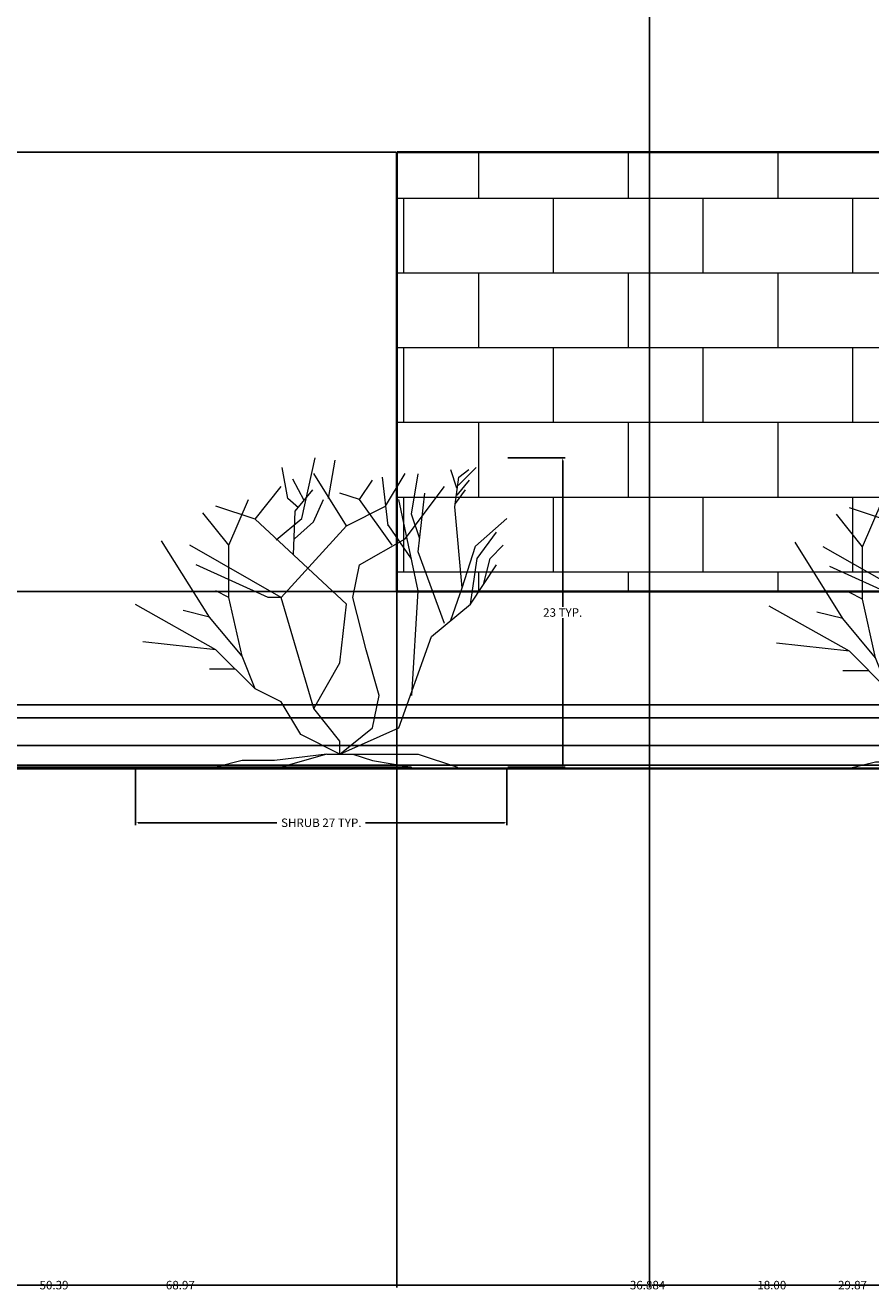
# Model space of a CAD drawing. Units: inches. Extents: x -13 to 809, y 112 to 656.
# Tile 2 of 55: x 49 to 111, y 112 to 205. Entities that reach past the tile are written whole.
import ezdxf

# ---------------------------------------------------------------- set-up
doc = ezdxf.new("R2010")
doc.units = ezdxf.units.IN
doc.header["$MEASUREMENT"] = 0
for name, color, linetype, lineweight in [('A-ANNO-DIMS', 2, 'Continuous', 18), ('A-ELEV', 7, 'Continuous', 35), ('A-ELEV-PATT', 8, 'Continuous', 13), ('L-PLNT', 3, 'Continuous', 18)]:
    doc.layers.add(name, color=color, linetype=linetype, lineweight=lineweight)
doc.styles.get("Standard").update_dxf_attribs({"font": 'arial.ttf'})
doc.dimstyles.get("Standard").update_dxf_attribs({"dimtxt": 0.625, "dimasz": 0.18, "dimexe": 0.18, "dimexo": 0.0625, "dimgap": 0.09, "dimtad": 0, "dimtih": 1, "dimtoh": 1, "dimdec": 4, "dimzin": 0, "dimdsep": 46, "dimlunit": 4, "dimtxsty": 'Standard', "dimcen": 0.09, "dimadec": 0, "dimazin": 0, "dimtfac": 1, "dimtdec": 4, "dimtofl": 0, "dimtmove": 0, "dimatfit": 3, "dimfxl": 1, "dimtolj": 1, "dimtzin": 0, "dimarcsym": 0})

# ---------------------------------------------------------------- blocks, each defined once
blk = doc.blocks.new('Shrub - elevation')
for p, q in [((-11.433, 18.289), (-10.457, 22.749)), ((-9.48, 19.775), (-8.992, 22.592)), ((-12.471, 19.775), (-12.898, 22.044)), ((-8.16, 17.76), (-10.56, 21.6)), ((-5.28, 19.2), (-3.84, 21.6)), ((-3.377, 18.602), (-2.888, 21.575)), ((-0.508, 21.888), (-0.081, 20.558)), ((0.041, 20.714), (1.384, 22.044)), ((0.102, 21.34), (0.835, 21.888)), ((-14.88, 18.24), (-12.96, 20.64)), ((-11.28, 19.619), (-12.104, 21.184)), ((-7.2, 19.68), (-6.24, 21.12)), ((-5.086, 17.741), (-5.513, 21.34)), ((-3.84, 16.8), (-0.96, 20.64)), ((-0.203, 19.149), (0.102, 21.34)), ((-0.02, 20.01), (0.896, 21.105)), ((-16.8, 16.32), (-15.36, 19.68)), ((-11.677, 19.071), (-12.471, 19.775)), ((-11.921, 18.836), (-10.64, 20.401)), ((-10.579, 18.054), (-9.846, 19.697)), ((-7.2, 19.68), (-8.64, 20.16)), ((-4.8, 16.32), (-7.2, 19.68)), ((-2.88, 12.96), (-4.32, 19.68)), ((-2.88, 15.84), (-2.4, 20.16)), ((-0.142, 19.384), (0.59, 20.401)), ((-16.8, 16.32), (-18.72, 18.72)), ((-14.88, 18.24), (-17.76, 19.2)), ((-12.043, 15.628), (-11.921, 18.836)), ((-8.16, 17.76), (-5.28, 19.2)), ((0.346, 13.203), (-0.203, 19.149)), ((-8.16, 12), (-14.88, 18.24)), ((-13.325, 16.724), (-11.433, 18.289)), ((-12.96, 12.48), (-8.16, 17.76)), ((-11.982, 16.802), (-10.579, 18.054)), ((-3.377, 15.315), (-5.086, 17.819)), ((-2.766, 16.802), (-3.377, 18.602)), ((1.323, 16.254), (3.642, 18.289)), ((-7.2, 14.88), (-3.84, 16.8)), ((1.44, 15.36), (2.88, 17.28)), ((-18.24, 11.04), (-21.755, 16.655)), ((-12.96, 12.48), (-19.68, 16.32)), ((-16.8, 12.48), (-16.8, 16.32)), ((-0.96, 10.56), (-2.88, 15.84)), ((0.346, 13.203), (1.323, 16.254)), ((2.4, 15.36), (3.36, 16.32)), ((0.96, 12), (1.44, 15.36)), ((1.92, 13.44), (2.4, 15.36)), ((-13.92, 12.48), (-19.2, 14.88)), ((-7.68, 12.48), (-7.2, 14.88)), ((0.96, 12), (2.88, 14.88)), ((-0.48, 10.8), (0.346, 13.203)), ((-16.8, 12.48), (-17.76, 12.96)), ((-15.84, 8.16), (-16.8, 12.48)), ((-12.96, 12.48), (-13.92, 12.48)), ((-10.56, 4.32), (-12.96, 12.48)), ((-6.72, 8.64), (-7.68, 12.48)), ((-3.36, 5.28), (-2.88, 12.96)), ((-17.76, 8.64), (-23.663, 11.961)), ((-18.24, 11.04), (-20.16, 11.52)), ((-8.64, 7.68), (-8.16, 12)), ((-1.92, 9.6), (0.96, 12)), ((-15.84, 8.16), (-18.24, 11.04)), ((-4.32, 2.88), (-1.92, 9.6)), ((-17.76, 8.64), (-23.128, 9.222)), ((-14.88, 5.76), (-17.76, 8.64)), ((-5.76, 5.28), (-6.72, 8.64)), ((-14.88, 5.76), (-15.84, 8.16)), ((-10.56, 4.32), (-8.64, 7.68)), ((-16.32, 7.2), (-18.24, 7.2)), ((-12.96, 4.8), (-14.88, 5.76)), ((-11.52, 2.4), (-12.96, 4.8)), ((-6.24, 2.88), (-5.76, 5.28)), ((-8.64, 1.92), (-10.56, 4.32)), ((-8.64, 0.96), (-4.32, 2.88)), ((-8.64, 0.96), (-6.24, 2.88)), ((-8.64, 0.96), (-11.52, 2.4)), ((-8.64, 0.96), (-8.64, 1.92)), ((-9.6, 0.96), (-13.44, 0.48)), ((-9.6, 0.96), (-12.96, 0)), ((-9.6, 0.96), (-7.68, 0.96)), ((-8.64, 0.96), (-2.88, 0.96)), ((-7.68, 0.96), (-6.24, 0.48)), ((-2.88, 0.96), (0, 0)), ((-15.84, 0.48), (-17.76, 0)), ((-13.44, 0.48), (-15.84, 0.48)), ((-6.24, 0.48), (-3.36, 0))]:
    blk.add_line(p, q)
blk = doc.blocks.new('*D7')
at = {"layer": 'A-ANNO-DIMS', "color": 0, "lineweight": -2, "transparency": 16777216}
for p, q in [((57.274, 150.572), (57.274, 146.359)), ((84.579, 150.572), (84.579, 146.359)), ((57.454, 146.539), (67.668, 146.539)), ((84.399, 146.539), (74.186, 146.539))]:
    blk.add_line(p, q, dxfattribs=at)
at = {"layer": 'A-ANNO-DIMS', "color": 0, "transparency": 16777216}
for points in [[(57.454, 146.569), (57.454, 146.509), (57.274, 146.539)], [(84.399, 146.569), (84.399, 146.509), (84.579, 146.539)]]:
    blk.add_solid(points, dxfattribs=at)
at = {"layer": 'Defpoints', "color": 0, "transparency": 16777216}
for p in [(57.274, 150.634), (84.579, 150.634), (84.579, 146.539)]:
    blk.add_point(p, dxfattribs=at)
at = {"layer": 'A-ANNO-DIMS', "color": 0, "transparency": 16777216, "insert": (70.927, 146.539), "char_height": 0.625, "attachment_point": 5}
blk.add_mtext('\\A1;SHRUB 27 TYP.', dxfattribs=at)
blk = doc.blocks.new('*D8')
at = {"layer": 'A-ANNO-DIMS', "color": 0, "lineweight": -2, "transparency": 16777216}
for p, q in [((84.642, 173.383), (88.855, 173.383)), ((88.675, 173.203), (88.675, 162.418)), ((88.675, 150.814), (88.675, 161.599)), ((84.642, 150.634), (88.855, 150.634))]:
    blk.add_line(p, q, dxfattribs=at)
at = {"layer": 'A-ANNO-DIMS', "color": 0, "transparency": 16777216}
for points in [[(88.645, 173.203), (88.705, 173.203), (88.675, 173.383)], [(88.645, 150.814), (88.705, 150.814), (88.675, 150.634)]]:
    blk.add_solid(points, dxfattribs=at)
at = {"layer": 'Defpoints', "color": 0, "transparency": 16777216}
for p in [(84.579, 173.383), (88.675, 173.383), (84.579, 150.634)]:
    blk.add_point(p, dxfattribs=at)
at = {"layer": 'A-ANNO-DIMS', "color": 0, "transparency": 16777216, "insert": (88.675, 162.009), "char_height": 0.625, "attachment_point": 5}
blk.add_mtext('\\A1;23 TYP.', dxfattribs=at)
blk = doc.blocks.new('*D11')
at = {"layer": 'A-ANNO-DIMS', "color": 0, "lineweight": -2, "transparency": 16777216}
for p, q in [((95.047, 306.457), (95.047, 112.34)), ((26.081, 150.457), (26.081, 112.34)), ((26.261, 112.52), (59.418, 112.52)), ((94.867, 112.52), (61.71, 112.52))]:
    blk.add_line(p, q, dxfattribs=at)
at = {"layer": 'A-ANNO-DIMS', "color": 0, "transparency": 16777216}
for points in [[(26.261, 112.55), (26.261, 112.49), (26.081, 112.52)], [(94.867, 112.55), (94.867, 112.49), (95.047, 112.52)]]:
    blk.add_solid(points, dxfattribs=at)
at = {"layer": 'Defpoints', "color": 0, "transparency": 16777216}
for p in [(95.047, 306.52), (26.081, 150.52), (95.047, 112.52)]:
    blk.add_point(p, dxfattribs=at)
at = {"layer": 'A-ANNO-DIMS', "color": 0, "transparency": 16777216, "insert": (60.564, 112.52), "char_height": 0.625, "attachment_point": 5}
blk.add_mtext('\\A1;68.97', dxfattribs=at)
blk = doc.blocks.new('*D12')
at = {"layer": 'A-ANNO-DIMS', "color": 0, "lineweight": -2, "transparency": 16777216}
for p, q in [((95.047, 306.457), (95.047, 112.34)), ((124.918, 210.457), (124.918, 112.34)), ((95.227, 112.52), (108.833, 112.52)), ((124.738, 112.52), (111.133, 112.52))]:
    blk.add_line(p, q, dxfattribs=at)
at = {"layer": 'A-ANNO-DIMS', "color": 0, "transparency": 16777216}
for points in [[(95.227, 112.55), (95.227, 112.49), (95.047, 112.52)], [(124.738, 112.55), (124.738, 112.49), (124.918, 112.52)]]:
    blk.add_solid(points, dxfattribs=at)
at = {"layer": 'Defpoints', "color": 0, "transparency": 16777216}
for p in [(95.047, 306.52), (124.918, 210.52), (124.918, 112.52)]:
    blk.add_point(p, dxfattribs=at)
at = {"layer": 'A-ANNO-DIMS', "color": 0, "transparency": 16777216, "insert": (109.983, 112.52), "char_height": 0.625, "attachment_point": 5}
blk.add_mtext('\\A1;29.87', dxfattribs=at)
blk = doc.blocks.new('*D85')
at = {"layer": 'A-ANNO-DIMS', "color": 0, "lineweight": -2, "transparency": 16777216}
for p, q in [((76.473, 195.828), (76.473, 112.34)), ((113.357, 195.828), (113.357, 112.34)), ((76.653, 112.52), (93.529, 112.52)), ((113.177, 112.52), (96.301, 112.52))]:
    blk.add_line(p, q, dxfattribs=at)
at = {"layer": 'A-ANNO-DIMS', "color": 0, "transparency": 16777216}
for points in [[(76.653, 112.55), (76.653, 112.49), (76.473, 112.52)], [(113.177, 112.55), (113.177, 112.49), (113.357, 112.52)]]:
    blk.add_solid(points, dxfattribs=at)
at = {"layer": 'Defpoints', "color": 0, "transparency": 16777216}
for p in [(76.473, 195.891), (113.357, 195.891), (113.357, 112.52)]:
    blk.add_point(p, dxfattribs=at)
at = {"layer": 'A-ANNO-DIMS', "color": 0, "transparency": 16777216, "insert": (94.915, 112.52), "char_height": 0.625, "attachment_point": 5}
blk.add_mtext('\\A1;36.884', dxfattribs=at)
blk = doc.blocks.new('*D90')
at = {"layer": 'A-ANNO-DIMS', "color": 0, "lineweight": -2, "transparency": 16777216}
for p, q in [((26.081, 210.457), (26.081, 112.34)), ((76.473, 195.828), (76.473, 112.34)), ((26.261, 112.52), (50.132, 112.52)), ((76.293, 112.52), (52.422, 112.52))]:
    blk.add_line(p, q, dxfattribs=at)
at = {"layer": 'A-ANNO-DIMS', "color": 0, "transparency": 16777216}
for points in [[(26.261, 112.55), (26.261, 112.49), (26.081, 112.52)], [(76.293, 112.55), (76.293, 112.49), (76.473, 112.52)]]:
    blk.add_solid(points, dxfattribs=at)
at = {"layer": 'Defpoints', "color": 0, "transparency": 16777216}
for p in [(26.081, 210.52), (76.473, 195.891), (76.473, 112.52)]:
    blk.add_point(p, dxfattribs=at)
at = {"layer": 'A-ANNO-DIMS', "color": 0, "transparency": 16777216, "insert": (51.277, 112.52), "char_height": 0.625, "attachment_point": 5}
blk.add_mtext('\\A1;50.39', dxfattribs=at)
blk = doc.blocks.new('*D91')
at = {"layer": 'A-ANNO-DIMS', "color": 0, "lineweight": -2, "transparency": 16777216}
for p, q in [((76.411, 163.564), (-12.099, 163.564)), ((-11.919, 163.384), (-11.919, 157.508)), ((-11.919, 150.814), (-11.919, 156.69)), ((77.515, 150.634), (-12.099, 150.634))]:
    blk.add_line(p, q, dxfattribs=at)
at = {"layer": 'A-ANNO-DIMS', "color": 0, "transparency": 16777216}
for points in [[(-11.949, 163.384), (-11.889, 163.384), (-11.919, 163.564)], [(-11.949, 150.814), (-11.889, 150.814), (-11.919, 150.634)]]:
    blk.add_solid(points, dxfattribs=at)
at = {"layer": 'Defpoints', "color": 0, "transparency": 16777216}
for p in [(-11.919, 163.564), (76.473, 163.564), (77.577, 150.634)]:
    blk.add_point(p, dxfattribs=at)
at = {"layer": 'A-ANNO-DIMS', "color": 0, "transparency": 16777216, "insert": (-11.919, 157.099), "char_height": 0.625, "attachment_point": 5}
blk.add_mtext('\\A1;12.93', dxfattribs=at)
blk = doc.blocks.new('*D92')
at = {"layer": 'A-ANNO-DIMS', "color": 0, "lineweight": -2, "transparency": 16777216}
for p, q in [((76.411, 195.891), (-12.099, 195.891)), ((-11.919, 195.711), (-11.919, 180.137)), ((-11.919, 163.744), (-11.919, 179.318)), ((76.411, 163.564), (-12.099, 163.564))]:
    blk.add_line(p, q, dxfattribs=at)
at = {"layer": 'A-ANNO-DIMS', "color": 0, "transparency": 16777216}
for points in [[(-11.949, 195.711), (-11.889, 195.711), (-11.919, 195.891)], [(-11.949, 163.744), (-11.889, 163.744), (-11.919, 163.564)]]:
    blk.add_solid(points, dxfattribs=at)
at = {"layer": 'Defpoints', "color": 0, "transparency": 16777216}
for p in [(-11.919, 195.891), (76.473, 195.891), (76.473, 163.564)]:
    blk.add_point(p, dxfattribs=at)
at = {"layer": 'A-ANNO-DIMS', "color": 0, "transparency": 16777216, "insert": (-11.919, 179.727), "char_height": 0.625, "attachment_point": 5}
blk.add_mtext('\\A1;32.33', dxfattribs=at)
blk = doc.blocks.new('*D107')
at = {"layer": 'A-ANNO-DIMS', "color": 0, "lineweight": -2, "transparency": 16777216}
for p, q in [((113.047, 324.457), (113.047, 112.34)), ((95.047, 306.457), (95.047, 112.34)), ((95.227, 112.52), (102.933, 112.52)), ((112.867, 112.52), (105.161, 112.52))]:
    blk.add_line(p, q, dxfattribs=at)
at = {"layer": 'A-ANNO-DIMS', "color": 0, "transparency": 16777216}
for points in [[(95.227, 112.55), (95.227, 112.49), (95.047, 112.52)], [(112.867, 112.55), (112.867, 112.49), (113.047, 112.52)]]:
    blk.add_solid(points, dxfattribs=at)
at = {"layer": 'Defpoints', "color": 0, "transparency": 16777216}
for p in [(113.047, 324.52), (95.047, 306.52), (113.047, 112.52)]:
    blk.add_point(p, dxfattribs=at)
at = {"layer": 'A-ANNO-DIMS', "color": 0, "transparency": 16777216, "insert": (104.047, 112.52), "char_height": 0.625, "attachment_point": 5}
blk.add_mtext('\\A1;18.00', dxfattribs=at)
blk = doc.blocks.new('*D115')
at = {"layer": 'A-ANNO-DIMS', "color": 0, "lineweight": -2, "transparency": 16777216}
for p, q in [((311.4, 210.785), (-12.099, 210.785)), ((-11.919, 210.605), (-11.919, 181.062)), ((-11.919, 150.7), (-11.919, 180.243)), ((311.637, 150.52), (-12.099, 150.52))]:
    blk.add_line(p, q, dxfattribs=at)
at = {"layer": 'A-ANNO-DIMS', "color": 0, "transparency": 16777216}
for points in [[(-11.949, 210.605), (-11.889, 210.605), (-11.919, 210.785)], [(-11.949, 150.7), (-11.889, 150.7), (-11.919, 150.52)]]:
    blk.add_solid(points, dxfattribs=at)
at = {"layer": 'Defpoints', "color": 0, "transparency": 16777216}
for p in [(-11.919, 210.785), (311.463, 210.785), (311.699, 150.52)]:
    blk.add_point(p, dxfattribs=at)
at = {"layer": 'A-ANNO-DIMS', "color": 0, "transparency": 16777216, "insert": (-11.919, 180.652), "char_height": 0.625, "attachment_point": 5}
blk.add_mtext('\\A1;60.27', dxfattribs=at)
blk = doc.blocks.new('*D117')
at = {"layer": 'A-ANNO-DIMS', "color": 0, "lineweight": -2, "transparency": 16777216}
for p, q in [((260.642, 154.272), (-12.099, 154.272)), ((-11.919, 154.092), (-11.919, 152.938)), ((-11.919, 150.965), (-11.919, 152.119)), ((258.04, 150.785), (-12.099, 150.785))]:
    blk.add_line(p, q, dxfattribs=at)
at = {"layer": 'A-ANNO-DIMS', "color": 0, "transparency": 16777216}
for points in [[(-11.949, 154.092), (-11.889, 154.092), (-11.919, 154.272)], [(-11.949, 150.965), (-11.889, 150.965), (-11.919, 150.785)]]:
    blk.add_solid(points, dxfattribs=at)
at = {"layer": 'Defpoints', "color": 0, "transparency": 16777216}
for p in [(260.705, 154.272), (-11.919, 150.785), (258.102, 150.785)]:
    blk.add_point(p, dxfattribs=at)
at = {"layer": 'A-ANNO-DIMS', "color": 0, "transparency": 16777216, "insert": (-11.919, 152.529), "char_height": 0.625, "attachment_point": 5}
blk.add_mtext('\\A1;3.487', dxfattribs=at)
blk = doc.blocks.new('*D131')
at = {"layer": 'A-ANNO-DIMS', "color": 0, "lineweight": -2, "transparency": 16777216}
for p, q in [((368.876, 155.214), (-12.099, 155.214)), ((-11.919, 155.034), (-11.919, 154.123)), ((-11.919, 152.394), (-11.919, 153.305)), ((365.876, 152.214), (-12.099, 152.214))]:
    blk.add_line(p, q, dxfattribs=at)
at = {"layer": 'A-ANNO-DIMS', "color": 0, "transparency": 16777216}
for points in [[(-11.949, 155.034), (-11.889, 155.034), (-11.919, 155.214)], [(-11.949, 152.394), (-11.889, 152.394), (-11.919, 152.214)]]:
    blk.add_solid(points, dxfattribs=at)
at = {"layer": 'Defpoints', "color": 0, "transparency": 16777216}
for p in [(368.938, 155.214), (-11.919, 152.214), (365.938, 152.214)]:
    blk.add_point(p, dxfattribs=at)
at = {"layer": 'A-ANNO-DIMS', "color": 0, "transparency": 16777216, "insert": (-11.919, 153.714), "char_height": 0.625, "attachment_point": 5}
blk.add_mtext('\\A1;3.00', dxfattribs=at)

msp = doc.modelspace()

# ---------------------------------------------------------------- hatches: boundary and pattern name
at = {"layer": 'A-ELEV-PATT'}
h = msp.add_hatch(dxfattribs=at)
h.set_pattern_fill('BRICK', color=256, scale=22)
h.paths.add_polyline_path([(113.3574, 195.8907), (76.4733, 195.8907), (76.4733, 163.5637), (113.3574, 163.5637)])
h.paths.add_polyline_path([(167.4098, 195.8907), (129.2551, 195.8907), (129.2551, 163.5637), (167.4098, 163.5637)])
h.paths.add_polyline_path([(229.6736, 195.8907), (184.0557, 195.8907), (184.0557, 163.5637), (229.6736, 163.5637)])

# ---------------------------------------------------------------- linework, layer by layer
at = {"layer": 'A-ELEV'}
for q in [(26.0809, 150.5199), (649.5888, 150.5199)]:
    msp.add_line((109.5888, 150.5199), q, dxfattribs=at)
msp.add_lwpolyline([(76.4733, 195.8907), (229.6736, 195.8907), (229.6736, 163.5637), (76.4733, 163.5637)], close=True, dxfattribs=at)

# ---------------------------------------------------------------- block references
at = {"layer": 'L-PLNT'}
for p in [(80.9373, 150.6343), (127.517, 150.5199)]:
    msp.add_blockref('Shrub - elevation', p, dxfattribs=at)

# ---------------------------------------------------------------- dimensions: what is measured, and where the dimension line sits
at = {"layer": 'A-ANNO-DIMS'}
for base, p1, p2, override, picture, middle in [((113.0469, 112.5199), (95.0469, 306.5199), (113.0469, 324.5199), {"dimdec": 2, "dimlfac": 1, "dimrnd": 0, "dimzin": 0, "dimdsep": 46, "dimlunit": 2}, '*D107', (104.0469, 112.5199)), ((95.0469, 112.5199), (26.0809, 150.5199), (95.0469, 306.5199), {"dimdec": 2, "dimlfac": 1, "dimrnd": 0, "dimzin": 0, "dimdsep": 46, "dimlunit": 2}, '*D11', (60.5639, 112.5199)), ((124.9184, 112.5199), (95.0469, 306.5199), (124.9184, 210.5199), {"dimdec": 2, "dimlfac": 1, "dimrnd": 0, "dimzin": 0, "dimdsep": 46, "dimlunit": 2}, '*D12', (109.9827, 112.5199)), ((76.4733, 112.5199), (26.0809, 210.5199), (76.4733, 195.8907), {"dimdec": 2, "dimlfac": 1, "dimrnd": 0, "dimzin": 0, "dimdsep": 46, "dimlunit": 2}, '*D90', (51.2771, 112.5199)), ((113.3574, 112.5199), (76.4733, 195.8907), (113.3574, 195.8907), {"dimdec": 3, "dimlfac": 1, "dimrnd": 0, "dimzin": 0, "dimdsep": 46, "dimlunit": 2}, '*D85', (94.9153, 112.5199))]:
    dim = msp.add_linear_dim(base=base, p1=p1, p2=p2, dimstyle='Standard', override=override, dxfattribs=at)
    dim.commit()
    dim.dimension.update_dxf_attribs({"geometry": picture, "text_midpoint": middle})
for base, p1, p2, override, picture, middle in [((-11.91915, 210.78493), (311.6991, 150.51989), (311.46269, 210.78493), {"dimdec": 2, "dimlfac": 1, "dimrnd": 0, "dimzin": 0, "dimdsep": 46, "dimlunit": 2}, '*D115', (-11.91915, 180.65241)), ((-11.9191, 195.8907), (76.4733, 163.5637), (76.4733, 195.8907), {"dimdec": 2, "dimlfac": 1, "dimrnd": 0, "dimzin": 0, "dimdsep": 46, "dimlunit": 2}, '*D92', (-11.9191, 179.7272)), ((-11.9191, 163.5637), (77.5773, 150.6343), (76.4733, 163.5637), {"dimdec": 2, "dimlfac": 1, "dimrnd": 0, "dimzin": 0, "dimdsep": 46, "dimlunit": 2}, '*D91', (-11.9191, 157.099)), ((-11.9191, 152.2141), (368.9383, 155.2141), (365.9383, 152.2141), {"dimdec": 2, "dimlfac": 1, "dimrnd": 0, "dimzin": 0, "dimdsep": 46, "dimlunit": 2}, '*D131', (-11.9191, 153.7141)), ((-11.9191, 150.7849), (260.7048, 154.2723), (258.1022, 150.7849), {"dimdec": 3, "dimlfac": 1, "dimrnd": 0, "dimzin": 0, "dimdsep": 46, "dimlunit": 2}, '*D117', (-11.9191, 152.5286))]:
    dim = msp.add_linear_dim(base=base, p1=p1, p2=p2, angle=90, dimstyle='Standard', override=override, dxfattribs=at)
    dim.commit()
    dim.dimension.update_dxf_attribs({"geometry": picture, "text_midpoint": middle})
dim = msp.add_linear_dim(base=(88.675, 173.3833), p1=(84.5793, 150.6343), p2=(84.5793, 173.3833), angle=90, text='<> TYP.', dimstyle='Standard', override={"dimdec": 0, "dimlfac": 1, "dimrnd": 0, "dimzin": 0, "dimdsep": 46, "dimlunit": 2}, dxfattribs=at)
dim.commit()
dim.dimension.update_dxf_attribs({"geometry": '*D8', "text_midpoint": (88.675, 162.0088)})
dim = msp.add_linear_dim(base=(84.5793, 146.5385), p1=(57.2743, 150.6343), p2=(84.5793, 150.6343), text='SHRUB <> TYP.', dimstyle='Standard', override={"dimdec": 0, "dimlfac": 1, "dimrnd": 0, "dimzin": 0, "dimdsep": 46, "dimlunit": 2}, dxfattribs=at)
dim.commit()
dim.dimension.update_dxf_attribs({"geometry": '*D7', "text_midpoint": (70.9268, 146.5385)})

doc.saveas('drawing.dxf')
